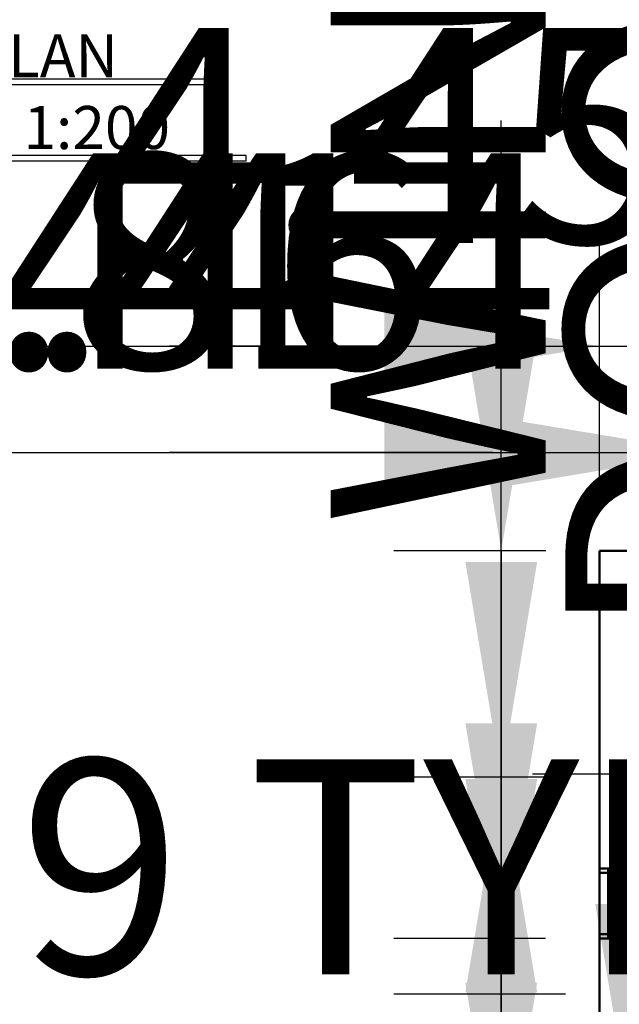
# Model space of a CAD drawing. Units: metres. Extents: x 782 to 1487, y 1262 to 7446.
# Tile 16 of 25: x 821.23 to 828.19, y 1302.06 to 1313.5. Entities that reach past the tile are written whole.
import ezdxf

# ---------------------------------------------------------------- set-up
doc = ezdxf.new("R2010")
doc.units = ezdxf.units.M
for name, color, linetype, lineweight in [('A-ANNO-DIMS', 2, 'Continuous', 18), ('A-ANNO-TEXT', 3, 'Continuous', 18), ('A-WALL', 7, 'Continuous', 50), ('C-PROP', 6, 'Continuous', 25)]:
    doc.layers.add(name, color=color, linetype=linetype, lineweight=lineweight)
doc.styles.get("Standard").update_dxf_attribs({"font": 'arial.ttf'})
doc.dimstyles.new('ISO-25', dxfattribs={"dimtxt": 2.5, "dimasz": 2.5, "dimexe": 1.25, "dimexo": 0.625, "dimtad": 1, "dimtxsty": 'Standard', "dimcen": 2.5, "dimadec": 0, "dimazin": 0, "dimtfac": 1, "dimtmove": 0, "dimatfit": 3, "dimfxl": 1, "dimarcsym": 0})

# ---------------------------------------------------------------- blocks, each defined once
blk = doc.blocks.new('*D5')
at = {"layer": 'A-ANNO-DIMS', "color": 0, "lineweight": -2, "transparency": 16777216}
for p, q in [((812.13, 1307.952), (812.13, 1310.955)), ((816.58, 1307.952), (816.58, 1310.955)), ((809.63, 1309.705), (807.13, 1309.705)), ((812.13, 1309.705), (816.58, 1309.705)), ((819.08, 1309.705), (829.443, 1309.705))]:
    blk.add_line(p, q, dxfattribs=at)
at = {"layer": 'A-ANNO-DIMS', "color": 0, "transparency": 16777216}
for points in [[(809.63, 1310.122), (809.63, 1309.289), (812.13, 1309.705)], [(819.08, 1310.122), (819.08, 1309.289), (816.58, 1309.705)]]:
    blk.add_solid(points, dxfattribs=at)
at = {"layer": 'Defpoints', "color": 0, "transparency": 16777216}
for p in [(816.58, 1309.705), (812.13, 1307.327), (816.58, 1307.327)]:
    blk.add_point(p, dxfattribs=at)
at = {"layer": 'A-ANNO-DIMS', "color": 0, "transparency": 16777216, "insert": (825.512, 1311.828), "char_height": 2.5, "attachment_point": 5}
blk.add_mtext('4,45', dxfattribs=at)
blk = doc.blocks.new('*D7')
at = {"layer": 'A-ANNO-DIMS', "color": 0, "lineweight": -2, "transparency": 16777216}
for p, q in [((827.962, 1307.952), (827.962, 1310.955)), ((832.412, 1307.952), (832.412, 1310.955)), ((825.462, 1309.705), (822.962, 1309.705)), ((827.962, 1309.705), (832.412, 1309.705)), ((834.912, 1309.705), (845.276, 1309.705))]:
    blk.add_line(p, q, dxfattribs=at)
at = {"layer": 'A-ANNO-DIMS', "color": 0, "transparency": 16777216}
for points in [[(825.462, 1310.122), (825.462, 1309.289), (827.962, 1309.705)], [(834.912, 1310.122), (834.912, 1309.289), (832.412, 1309.705)]]:
    blk.add_solid(points, dxfattribs=at)
at = {"layer": 'Defpoints', "color": 0, "transparency": 16777216}
for p in [(832.412, 1309.705), (827.962, 1307.327), (832.412, 1307.327)]:
    blk.add_point(p, dxfattribs=at)
at = {"layer": 'A-ANNO-DIMS', "color": 0, "transparency": 16777216, "insert": (841.344, 1311.828), "char_height": 2.5, "attachment_point": 5}
blk.add_mtext('4,45', dxfattribs=at)
blk = doc.blocks.new('*D20')
at = {"layer": 'A-ANNO-DIMS', "color": 0, "lineweight": -2, "transparency": 16777216}
for p, q in [((831.056, 1302.088), (831.056, 1337.678)), ((831.056, 1298.698), (831.056, 1299.588)), ((831.548, 1299.588), (832.306, 1299.588)), ((831.548, 1298.698), (832.306, 1298.698)), ((831.056, 1296.198), (831.056, 1293.698))]:
    blk.add_line(p, q, dxfattribs=at)
at = {"layer": 'A-ANNO-DIMS', "color": 0, "transparency": 16777216}
for points in [[(830.64, 1302.088), (831.473, 1302.088), (831.056, 1299.588)], [(830.64, 1296.198), (831.473, 1296.198), (831.056, 1298.698)]]:
    blk.add_solid(points, dxfattribs=at)
at = {"layer": 'Defpoints', "color": 0, "transparency": 16777216}
for p in [(830.923, 1299.588), (831.056, 1299.588), (830.923, 1298.698)]:
    blk.add_point(p, dxfattribs=at)
at = {"layer": 'A-ANNO-DIMS', "color": 0, "transparency": 16777216, "insert": (829.138, 1321.133), "char_height": 2.5, "attachment_point": 5, "rotation": 90}
blk.add_mtext('DOOR D1 0.89 TYP.', dxfattribs=at)
blk = doc.blocks.new('*D21')
at = {"layer": 'A-ANNO-DIMS', "color": 0, "lineweight": -2, "transparency": 16777216}
for p, q in [((827.576, 1298.565), (825.076, 1298.565)), ((830.076, 1298.565), (830.923, 1298.565)), ((833.423, 1298.565), (852.255, 1298.565)), ((830.076, 1298.073), (830.076, 1297.315)), ((830.923, 1298.073), (830.923, 1297.315))]:
    blk.add_line(p, q, dxfattribs=at)
at = {"layer": 'A-ANNO-DIMS', "color": 0, "transparency": 16777216}
for points in [[(827.576, 1298.981), (827.576, 1298.148), (830.076, 1298.565)], [(833.423, 1298.981), (833.423, 1298.148), (830.923, 1298.565)]]:
    blk.add_solid(points, dxfattribs=at)
at = {"layer": 'Defpoints', "color": 0, "transparency": 16777216}
for p in [(830.076, 1298.698), (830.923, 1298.698), (830.923, 1298.565)]:
    blk.add_point(p, dxfattribs=at)
at = {"layer": 'A-ANNO-DIMS', "color": 0, "transparency": 16777216, "insert": (844.089, 1300.466), "char_height": 2.5, "attachment_point": 5}
blk.add_mtext('0.85 TYP.', dxfattribs=at)
blk = doc.blocks.new('*D24')
at = {"layer": 'A-ANNO-DIMS', "color": 0, "lineweight": -2, "transparency": 16777216}
for p, q in [((811.209, 1294.423), (808.709, 1294.423)), ((813.709, 1294.423), (814.559, 1294.423)), ((817.059, 1294.423), (852.649, 1294.423)), ((813.709, 1293.926), (813.709, 1293.173)), ((814.559, 1293.926), (814.559, 1293.173))]:
    blk.add_line(p, q, dxfattribs=at)
at = {"layer": 'A-ANNO-DIMS', "color": 0, "transparency": 16777216}
for points in [[(811.209, 1294.84), (811.209, 1294.006), (813.709, 1294.423)], [(817.059, 1294.84), (817.059, 1294.006), (814.559, 1294.423)]]:
    blk.add_solid(points, dxfattribs=at)
at = {"layer": 'Defpoints', "color": 0, "transparency": 16777216}
for p in [(813.709, 1294.551), (814.559, 1294.551), (814.559, 1294.423)]:
    blk.add_point(p, dxfattribs=at)
at = {"layer": 'A-ANNO-DIMS', "color": 0, "transparency": 16777216, "insert": (836.104, 1296.342), "char_height": 2.5, "attachment_point": 5}
blk.add_mtext('DOOR D2 0.85 TYP.', dxfattribs=at)
blk = doc.blocks.new('*D26')
at = {"layer": 'A-ANNO-DIMS', "color": 0, "lineweight": -2, "transparency": 16777216}
for p, q in [((828.33, 1303.223), (828.33, 1342.718)), ((828.33, 1299.809), (828.33, 1300.723)), ((828.818, 1300.723), (829.58, 1300.723)), ((828.818, 1299.809), (829.58, 1299.809)), ((828.33, 1297.309), (828.33, 1294.809))]:
    blk.add_line(p, q, dxfattribs=at)
at = {"layer": 'A-ANNO-DIMS', "color": 0, "transparency": 16777216}
for points in [[(827.913, 1303.223), (828.747, 1303.223), (828.33, 1300.723)], [(827.913, 1297.309), (828.747, 1297.309), (828.33, 1299.809)]]:
    blk.add_solid(points, dxfattribs=at)
at = {"layer": 'Defpoints', "color": 0, "transparency": 16777216}
for p in [(828.193, 1300.723), (828.33, 1300.723), (828.193, 1299.809)]:
    blk.add_point(p, dxfattribs=at)
at = {"layer": 'A-ANNO-DIMS', "color": 0, "transparency": 16777216, "insert": (826.412, 1324.22), "char_height": 2.5, "attachment_point": 5, "rotation": 90}
blk.add_mtext('WINDOW W 0.91 TYP.', dxfattribs=at)
blk = doc.blocks.new('*D27')
at = {"layer": 'A-ANNO-DIMS', "color": 0, "lineweight": -2, "transparency": 16777216}
for p, q in [((825.463, 1299.672), (822.963, 1299.672)), ((827.963, 1299.672), (828.193, 1299.672)), ((830.693, 1299.672), (849.525, 1299.672)), ((827.963, 1299.184), (827.963, 1298.422)), ((828.193, 1299.184), (828.193, 1298.422))]:
    blk.add_line(p, q, dxfattribs=at)
at = {"layer": 'A-ANNO-DIMS', "color": 0, "transparency": 16777216}
for points in [[(825.463, 1300.088), (825.463, 1299.255), (827.963, 1299.672)], [(830.693, 1300.088), (830.693, 1299.255), (828.193, 1299.672)]]:
    blk.add_solid(points, dxfattribs=at)
at = {"layer": 'Defpoints', "color": 0, "transparency": 16777216}
for p in [(827.963, 1299.809), (828.193, 1299.809), (828.193, 1299.672)]:
    blk.add_point(p, dxfattribs=at)
at = {"layer": 'A-ANNO-DIMS', "color": 0, "transparency": 16777216, "insert": (841.359, 1301.574), "char_height": 2.5, "attachment_point": 5}
blk.add_mtext('0.23 TYP.', dxfattribs=at)
blk = doc.blocks.new('*D28')
at = {"layer": 'A-ANNO-DIMS', "color": 0, "lineweight": -2, "transparency": 16777216}
for p, q in [((832.55, 1308.281), (832.55, 1349.718)), ((832.55, 1304.867), (832.55, 1305.781)), ((833.038, 1305.781), (833.8, 1305.781)), ((833.038, 1304.867), (833.8, 1304.867)), ((832.55, 1302.367), (832.55, 1299.867))]:
    blk.add_line(p, q, dxfattribs=at)
at = {"layer": 'A-ANNO-DIMS', "color": 0, "transparency": 16777216}
for points in [[(832.134, 1308.281), (832.967, 1308.281), (832.55, 1305.781)], [(832.134, 1302.367), (832.967, 1302.367), (832.55, 1304.867)]]:
    blk.add_solid(points, dxfattribs=at)
at = {"layer": 'Defpoints', "color": 0, "transparency": 16777216}
for p in [(832.413, 1305.781), (832.55, 1305.781), (832.413, 1304.867)]:
    blk.add_point(p, dxfattribs=at)
at = {"layer": 'A-ANNO-DIMS', "color": 0, "transparency": 16777216, "insert": (830.632, 1330.25), "char_height": 2.5, "attachment_point": 5, "rotation": 90}
blk.add_mtext('WINDOW W1 0.91 TYP.', dxfattribs=at)
blk = doc.blocks.new('*D29')
at = {"layer": 'A-ANNO-DIMS', "color": 0, "lineweight": -2, "transparency": 16777216}
for p, q in [((829.683, 1304.73), (827.183, 1304.73)), ((832.183, 1304.73), (832.413, 1304.73)), ((834.913, 1304.73), (853.745, 1304.73)), ((832.183, 1304.242), (832.183, 1303.48)), ((832.413, 1304.242), (832.413, 1303.48))]:
    blk.add_line(p, q, dxfattribs=at)
at = {"layer": 'A-ANNO-DIMS', "color": 0, "transparency": 16777216}
for points in [[(829.683, 1305.146), (829.683, 1304.313), (832.183, 1304.73)], [(834.913, 1305.146), (834.913, 1304.313), (832.413, 1304.73)]]:
    blk.add_solid(points, dxfattribs=at)
at = {"layer": 'Defpoints', "color": 0, "transparency": 16777216}
for p in [(832.183, 1304.867), (832.413, 1304.867), (832.413, 1304.73)]:
    blk.add_point(p, dxfattribs=at)
at = {"layer": 'A-ANNO-DIMS', "color": 0, "transparency": 16777216, "insert": (845.579, 1306.632), "char_height": 2.5, "attachment_point": 5}
blk.add_mtext('0.23 TYP.', dxfattribs=at)
blk = doc.blocks.new('*D30')
at = {"layer": 'A-ANNO-DIMS', "color": 0, "lineweight": -2, "transparency": 16777216}
for p, q in [((792.059, 1301.411), (789.559, 1301.411)), ((794.559, 1301.411), (794.946, 1301.411)), ((797.446, 1301.411), (832.354, 1301.411)), ((794.559, 1300.844), (794.559, 1300.161)), ((794.946, 1300.844), (794.946, 1300.161))]:
    blk.add_line(p, q, dxfattribs=at)
at = {"layer": 'A-ANNO-DIMS', "color": 0, "transparency": 16777216}
for points in [[(792.059, 1301.827), (792.059, 1300.994), (794.559, 1301.411)], [(797.446, 1301.827), (797.446, 1300.994), (794.946, 1301.411)]]:
    blk.add_solid(points, dxfattribs=at)
at = {"layer": 'Defpoints', "color": 0, "transparency": 16777216}
for p in [(794.559, 1301.469), (794.946, 1301.469), (794.946, 1301.411)]:
    blk.add_point(p, dxfattribs=at)
at = {"layer": 'A-ANNO-DIMS', "color": 0, "transparency": 16777216, "insert": (816.15, 1303.33), "char_height": 2.5, "attachment_point": 5}
blk.add_mtext('COLUMN 0.39 TYP.', dxfattribs=at)
blk = doc.blocks.new('*D70')
at = {"layer": 'A-ANNO-DIMS', "color": 0, "lineweight": -2, "transparency": 16777216}
for p, q in [((812.13, 1307.952), (812.13, 1309.718)), ((812.573, 1307.953), (812.573, 1309.718)), ((809.63, 1308.468), (807.13, 1308.468)), ((812.13, 1308.468), (812.573, 1308.468)), ((815.073, 1308.468), (825.307, 1308.468))]:
    blk.add_line(p, q, dxfattribs=at)
at = {"layer": 'A-ANNO-DIMS', "color": 0, "transparency": 16777216}
for points in [[(809.63, 1308.884), (809.63, 1308.051), (812.13, 1308.468)], [(815.073, 1308.884), (815.073, 1308.051), (812.573, 1308.468)]]:
    blk.add_solid(points, dxfattribs=at)
at = {"layer": 'Defpoints', "color": 0, "transparency": 16777216}
for p in [(812.573, 1308.468), (812.13, 1307.327), (812.573, 1307.328)]:
    blk.add_point(p, dxfattribs=at)
at = {"layer": 'A-ANNO-DIMS', "color": 0, "transparency": 16777216, "insert": (821.44, 1310.369), "char_height": 2.5, "attachment_point": 5}
blk.add_mtext('0.44', dxfattribs=at)
blk = doc.blocks.new('*D71')
at = {"layer": 'A-ANNO-DIMS', "color": 0, "lineweight": -2, "transparency": 16777216}
for p, q in [((812.573, 1307.953), (812.573, 1309.718)), ((813.387, 1307.953), (813.387, 1309.718)), ((810.073, 1308.468), (807.573, 1308.468)), ((812.573, 1308.468), (813.387, 1308.468)), ((815.887, 1308.468), (828.063, 1308.468))]:
    blk.add_line(p, q, dxfattribs=at)
at = {"layer": 'A-ANNO-DIMS', "color": 0, "transparency": 16777216}
for points in [[(810.073, 1308.884), (810.073, 1308.051), (812.573, 1308.468)], [(815.887, 1308.884), (815.887, 1308.051), (813.387, 1308.468)]]:
    blk.add_solid(points, dxfattribs=at)
at = {"layer": 'Defpoints', "color": 0, "transparency": 16777216}
for p in [(813.387, 1308.468), (812.573, 1307.328), (813.387, 1307.328)]:
    blk.add_point(p, dxfattribs=at)
at = {"layer": 'A-ANNO-DIMS', "color": 0, "transparency": 16777216, "insert": (823.225, 1310.369), "char_height": 2.5, "attachment_point": 5}
blk.add_mtext('0.814', dxfattribs=at)
blk = doc.blocks.new('*D72')
at = {"layer": 'A-ANNO-DIMS', "color": 0, "lineweight": -2, "transparency": 16777216}
for p, q in [((813.387, 1307.953), (813.387, 1309.718)), ((813.85, 1307.722), (813.85, 1309.718)), ((810.887, 1308.468), (808.387, 1308.468)), ((813.387, 1308.468), (813.85, 1308.468)), ((816.35, 1308.468), (826.592, 1308.468))]:
    blk.add_line(p, q, dxfattribs=at)
at = {"layer": 'A-ANNO-DIMS', "color": 0, "transparency": 16777216}
for points in [[(810.887, 1308.884), (810.887, 1308.051), (813.387, 1308.468)], [(816.35, 1308.884), (816.35, 1308.051), (813.85, 1308.468)]]:
    blk.add_solid(points, dxfattribs=at)
at = {"layer": 'Defpoints', "color": 0, "transparency": 16777216}
for p in [(813.85, 1308.468), (813.387, 1307.328), (813.85, 1307.097)]:
    blk.add_point(p, dxfattribs=at)
at = {"layer": 'A-ANNO-DIMS', "color": 0, "transparency": 16777216, "insert": (822.721, 1310.369), "char_height": 2.5, "attachment_point": 5}
blk.add_mtext('0.46', dxfattribs=at)
blk = doc.blocks.new('*D77')
at = {"layer": 'A-ANNO-DIMS', "color": 0, "lineweight": -2, "transparency": 16777216}
for p, q in [((826.821, 1309.827), (826.821, 1312.327)), ((827.337, 1307.327), (825.571, 1307.327)), ((826.821, 1307.327), (826.821, 1304.697)), ((827.567, 1304.697), (825.571, 1304.697)), ((826.821, 1302.197), (826.821, 1291.911))]:
    blk.add_line(p, q, dxfattribs=at)
at = {"layer": 'A-ANNO-DIMS', "color": 0, "transparency": 16777216}
for points in [[(826.404, 1309.827), (827.238, 1309.827), (826.821, 1307.327)], [(826.404, 1302.197), (827.238, 1302.197), (826.821, 1304.697)]]:
    blk.add_solid(points, dxfattribs=at)
at = {"layer": 'Defpoints', "color": 0, "transparency": 16777216}
for p in [(827.962, 1307.327), (826.821, 1304.697), (828.192, 1304.697)]:
    blk.add_point(p, dxfattribs=at)
at = {"layer": 'A-ANNO-DIMS', "color": 0, "transparency": 16777216, "insert": (824.919, 1295.804), "char_height": 2.5, "attachment_point": 5, "rotation": 90}
blk.add_mtext('2.63', dxfattribs=at)
blk = doc.blocks.new('*D78')
at = {"layer": 'A-ANNO-DIMS', "color": 0, "lineweight": -2, "transparency": 16777216}
for p, q in [((826.821, 1307.197), (826.821, 1309.697)), ((827.567, 1304.697), (825.571, 1304.697)), ((826.821, 1304.697), (826.821, 1302.822)), ((827.336, 1302.822), (825.571, 1302.822)), ((826.821, 1300.322), (826.821, 1290.308))]:
    blk.add_line(p, q, dxfattribs=at)
at = {"layer": 'A-ANNO-DIMS', "color": 0, "transparency": 16777216}
for points in [[(826.404, 1307.197), (827.238, 1307.197), (826.821, 1304.697)], [(826.404, 1300.322), (827.238, 1300.322), (826.821, 1302.822)]]:
    blk.add_solid(points, dxfattribs=at)
at = {"layer": 'Defpoints', "color": 0, "transparency": 16777216}
for p in [(828.192, 1304.697), (826.821, 1302.822), (827.961, 1302.822)]:
    blk.add_point(p, dxfattribs=at)
at = {"layer": 'A-ANNO-DIMS', "color": 0, "transparency": 16777216, "insert": (824.919, 1294.065), "char_height": 2.5, "attachment_point": 5, "rotation": 90}
blk.add_mtext('1.88', dxfattribs=at)
blk = doc.blocks.new('*D79')
at = {"layer": 'A-ANNO-DIMS', "color": 0, "lineweight": -2, "transparency": 16777216}
for p, q in [((826.821, 1305.322), (826.821, 1307.822)), ((827.336, 1302.822), (825.571, 1302.822)), ((826.821, 1302.822), (826.821, 1302.177)), ((827.567, 1302.177), (825.571, 1302.177)), ((826.821, 1299.677), (826.821, 1289.444))]:
    blk.add_line(p, q, dxfattribs=at)
at = {"layer": 'A-ANNO-DIMS', "color": 0, "transparency": 16777216}
for points in [[(826.404, 1305.322), (827.238, 1305.322), (826.821, 1302.822)], [(826.404, 1299.677), (827.238, 1299.677), (826.821, 1302.177)]]:
    blk.add_solid(points, dxfattribs=at)
at = {"layer": 'Defpoints', "color": 0, "transparency": 16777216}
for p in [(827.961, 1302.822), (826.821, 1302.177), (828.192, 1302.177)]:
    blk.add_point(p, dxfattribs=at)
at = {"layer": 'A-ANNO-DIMS', "color": 0, "transparency": 16777216, "insert": (824.919, 1293.311), "char_height": 2.5, "attachment_point": 5, "rotation": 90}
blk.add_mtext('0.64', dxfattribs=at)
blk = doc.blocks.new('*D80')
at = {"layer": 'A-ANNO-DIMS', "color": 0, "lineweight": -2, "transparency": 16777216}
for p, q in [((826.821, 1304.677), (826.821, 1307.177)), ((827.567, 1302.177), (825.571, 1302.177)), ((826.821, 1302.177), (826.821, 1299.809)), ((827.338, 1299.809), (825.571, 1299.809)), ((826.821, 1297.309), (826.821, 1287.022))]:
    blk.add_line(p, q, dxfattribs=at)
at = {"layer": 'A-ANNO-DIMS', "color": 0, "transparency": 16777216}
for points in [[(826.404, 1304.677), (827.238, 1304.677), (826.821, 1302.177)], [(826.404, 1297.309), (827.238, 1297.309), (826.821, 1299.809)]]:
    blk.add_solid(points, dxfattribs=at)
at = {"layer": 'Defpoints', "color": 0, "transparency": 16777216}
for p in [(828.192, 1302.177), (826.821, 1299.809), (827.963, 1299.809)]:
    blk.add_point(p, dxfattribs=at)
at = {"layer": 'A-ANNO-DIMS', "color": 0, "transparency": 16777216, "insert": (824.919, 1290.916), "char_height": 2.5, "attachment_point": 5, "rotation": 90}
blk.add_mtext('2.37', dxfattribs=at)
blk = doc.blocks.new('*D81')
at = {"layer": 'A-ANNO-DIMS', "color": 0, "lineweight": -2, "transparency": 16777216}
for p, q in [((826.821, 1302.309), (826.821, 1304.809)), ((827.338, 1299.809), (825.571, 1299.809)), ((826.821, 1299.809), (826.821, 1298.647)), ((827.567, 1298.647), (825.571, 1298.647)), ((826.821, 1296.147), (826.821, 1286.141))]:
    blk.add_line(p, q, dxfattribs=at)
at = {"layer": 'A-ANNO-DIMS', "color": 0, "transparency": 16777216}
for points in [[(826.404, 1302.309), (827.238, 1302.309), (826.821, 1299.809)], [(826.404, 1296.147), (827.238, 1296.147), (826.821, 1298.647)]]:
    blk.add_solid(points, dxfattribs=at)
at = {"layer": 'Defpoints', "color": 0, "transparency": 16777216}
for p in [(827.963, 1299.809), (826.821, 1298.647), (828.192, 1298.647)]:
    blk.add_point(p, dxfattribs=at)
at = {"layer": 'A-ANNO-DIMS', "color": 0, "transparency": 16777216, "insert": (824.919, 1289.894), "char_height": 2.5, "attachment_point": 5, "rotation": 90}
blk.add_mtext('1.16', dxfattribs=at)
blk = doc.blocks.new('*D82')
at = {"layer": 'A-ANNO-DIMS', "color": 0, "lineweight": -2, "transparency": 16777216}
for p, q in [((826.821, 1301.147), (826.821, 1303.647)), ((827.567, 1298.647), (825.571, 1298.647)), ((826.821, 1298.647), (826.821, 1296.5)), ((827.339, 1296.5), (825.571, 1296.5)), ((826.821, 1294), (826.821, 1281.772))]:
    blk.add_line(p, q, dxfattribs=at)
at = {"layer": 'A-ANNO-DIMS', "color": 0, "transparency": 16777216}
for points in [[(826.404, 1301.147), (827.238, 1301.147), (826.821, 1298.647)], [(826.404, 1294), (827.238, 1294), (826.821, 1296.5)]]:
    blk.add_solid(points, dxfattribs=at)
at = {"layer": 'Defpoints', "color": 0, "transparency": 16777216}
for p in [(828.192, 1298.647), (826.821, 1296.5), (827.964, 1296.5)]:
    blk.add_point(p, dxfattribs=at)
at = {"layer": 'A-ANNO-DIMS', "color": 0, "transparency": 16777216, "insert": (824.941, 1286.636), "char_height": 2.5, "attachment_point": 5, "rotation": 90}
blk.add_mtext('2.147', dxfattribs=at)
blk = doc.blocks.new('*D94')
at = {"layer": 'A-ANNO-DIMS', "color": 0, "lineweight": -2, "transparency": 16777216}
for p, q in [((827.962, 1307.952), (827.962, 1309.718)), ((828.406, 1307.953), (828.406, 1309.718)), ((825.462, 1308.468), (822.962, 1308.468)), ((827.962, 1308.468), (828.406, 1308.468)), ((830.906, 1308.468), (841.139, 1308.468))]:
    blk.add_line(p, q, dxfattribs=at)
at = {"layer": 'A-ANNO-DIMS', "color": 0, "transparency": 16777216}
for points in [[(825.462, 1308.884), (825.462, 1308.051), (827.962, 1308.468)], [(830.906, 1308.884), (830.906, 1308.051), (828.406, 1308.468)]]:
    blk.add_solid(points, dxfattribs=at)
at = {"layer": 'Defpoints', "color": 0, "transparency": 16777216}
for p in [(828.406, 1308.468), (827.962, 1307.327), (828.406, 1307.328)]:
    blk.add_point(p, dxfattribs=at)
at = {"layer": 'A-ANNO-DIMS', "color": 0, "transparency": 16777216, "insert": (837.273, 1310.369), "char_height": 2.5, "attachment_point": 5}
blk.add_mtext('0.44', dxfattribs=at)
blk = doc.blocks.new('*D95')
at = {"layer": 'A-ANNO-DIMS', "color": 0, "lineweight": -2, "transparency": 16777216}
for p, q in [((828.406, 1307.953), (828.406, 1309.718)), ((829.22, 1307.953), (829.22, 1309.718)), ((825.906, 1308.468), (823.406, 1308.468)), ((828.406, 1308.468), (829.22, 1308.468)), ((831.72, 1308.468), (843.896, 1308.468))]:
    blk.add_line(p, q, dxfattribs=at)
at = {"layer": 'A-ANNO-DIMS', "color": 0, "transparency": 16777216}
for points in [[(825.906, 1308.884), (825.906, 1308.051), (828.406, 1308.468)], [(831.72, 1308.884), (831.72, 1308.051), (829.22, 1308.468)]]:
    blk.add_solid(points, dxfattribs=at)
at = {"layer": 'Defpoints', "color": 0, "transparency": 16777216}
for p in [(829.22, 1308.468), (828.406, 1307.328), (829.22, 1307.328)]:
    blk.add_point(p, dxfattribs=at)
at = {"layer": 'A-ANNO-DIMS', "color": 0, "transparency": 16777216, "insert": (839.058, 1310.369), "char_height": 2.5, "attachment_point": 5}
blk.add_mtext('0.814', dxfattribs=at)
blk = doc.blocks.new('*D96')
at = {"layer": 'A-ANNO-DIMS', "color": 0, "lineweight": -2, "transparency": 16777216}
for p, q in [((829.22, 1307.953), (829.22, 1309.718)), ((829.682, 1307.722), (829.682, 1309.718)), ((826.72, 1308.468), (824.22, 1308.468)), ((829.22, 1308.468), (829.682, 1308.468)), ((832.182, 1308.468), (842.425, 1308.468))]:
    blk.add_line(p, q, dxfattribs=at)
at = {"layer": 'A-ANNO-DIMS', "color": 0, "transparency": 16777216}
for points in [[(826.72, 1308.884), (826.72, 1308.051), (829.22, 1308.468)], [(832.182, 1308.884), (832.182, 1308.051), (829.682, 1308.468)]]:
    blk.add_solid(points, dxfattribs=at)
at = {"layer": 'Defpoints', "color": 0, "transparency": 16777216}
for p in [(829.682, 1308.468), (829.22, 1307.328), (829.682, 1307.097)]:
    blk.add_point(p, dxfattribs=at)
at = {"layer": 'A-ANNO-DIMS', "color": 0, "transparency": 16777216, "insert": (838.554, 1310.369), "char_height": 2.5, "attachment_point": 5}
blk.add_mtext('0.46', dxfattribs=at)

msp = doc.modelspace()

# ---------------------------------------------------------------- linework, layer by layer
at = {"layer": 'A-WALL'}
for p, q in [((827.9625, 1304.6974), (827.9625, 1307.3274)), ((827.9625, 1307.3274), (829.4525, 1307.3274)), ((827.9625, 1302.1774), (827.9625, 1304.6974)), ((827.9609, 1302.8221), (827.9609, 1303.6361)), ((827.9609, 1303.6361), (828.1909, 1303.6361)), ((827.9609, 1303.6361), (827.9609, 1303.5853)), ((828.0632, 1303.6361), (828.0632, 1302.8221)), ((828.1909, 1303.6361), (828.0759, 1303.6361)), ((828.0759, 1303.6361), (828.0759, 1302.8221)), ((828.0886, 1303.6361), (828.0886, 1302.8221)), ((828.1909, 1303.6361), (828.1909, 1302.8221)), ((827.9609, 1303.5853), (828.1909, 1303.5853)), ((827.9609, 1302.8221), (827.9609, 1302.8729)), ((827.9609, 1302.8729), (828.1909, 1302.8729)), ((828.1909, 1302.8221), (827.9609, 1302.8221)), ((827.9625, 1298.6474), (827.9625, 1302.1774))]:
    msp.add_line(p, q, dxfattribs=at)
at = {"layer": 'C-PROP'}
for p, q in [((818.4097, 1312.8097), (823.558, 1312.8097)), ((823.558, 1312.8097), (823.558, 1312.7398)), ((823.558, 1312.7398), (818.4097, 1312.7398)), ((818.7034, 1311.923), (823.8517, 1311.923)), ((823.8517, 1311.8532), (818.7034, 1311.8532)), ((823.8517, 1311.923), (823.8517, 1311.8532))]:
    msp.add_line(p, q, dxfattribs=at)

# ---------------------------------------------------------------- texts
at = {"layer": 'A-ANNO-TEXT', "insert": (819.087, 1314.1616), "char_height": 0.5, "attachment_point": 1}
msp.add_mtext_dynamic_manual_height_columns('\\PSITE PLAN\\PSCALE 1:200', width=6.191207, gutter_width=12.5, heights=[0], dxfattribs=at)

# ---------------------------------------------------------------- dimensions: what is measured, and where the dimension line sits
at = {"layer": 'A-ANNO-DIMS'}
for base, p1, p2, text, picture, middle in [((832.5503, 1305.7809), (832.4132, 1304.8669), (832.4132, 1305.7809), 'WINDOW W1 <> TYP.', '*D28', (830.6318, 1330.2497)), ((828.3302, 1300.7228), (828.1931, 1299.8088), (828.1931, 1300.7228), 'WINDOW W <> TYP.', '*D26', (826.4117, 1324.2204)), ((831.0564, 1299.5877), (830.923, 1298.6982), (830.923, 1299.5877), 'DOOR D1 <> TYP.', '*D20', (829.138, 1321.1327))]:
    dim = msp.add_linear_dim(base=base, p1=p1, p2=p2, angle=90, text=text, dimstyle='ISO-25', override={"dimdec": 2, "dimlfac": 1, "dimrnd": 0, "dimzin": 0, "dimdsep": 46, "dimlunit": 2}, dxfattribs=at)
    dim.commit()
    dim.dimension.update_dxf_attribs({"geometry": picture, "text_midpoint": middle})
for base, p1, p2, override, picture, middle in [((816.58, 1309.7054), (812.13, 1307.3274), (816.58, 1307.3274), {"dimclrd": 0, "dimclre": 0, "dimclrt": 0}, '*D5', (825.5116, 1311.8277)), ((832.4125, 1309.7054), (827.9625, 1307.3274), (832.4125, 1307.3274), {"dimclrd": 0, "dimclre": 0, "dimclrt": 0}, '*D7', (841.3441, 1311.8277)), ((812.5733, 1308.4676), (812.13, 1307.3274), (812.5733, 1307.3276), {"dimdec": 2, "dimlfac": 1, "dimrnd": 0, "dimzin": 0, "dimdsep": 46, "dimlunit": 2}, '*D70', (821.4401, 1310.369)), ((813.3873, 1308.4676), (812.5733, 1307.3276), (813.3873, 1307.3276), {"dimdec": 3, "dimlfac": 1, "dimrnd": 0, "dimzin": 0, "dimdsep": 46, "dimlunit": 2}, '*D71', (823.2253, 1310.369)), ((813.85, 1308.4676), (813.3873, 1307.3276), (813.85, 1307.0974), {"dimdec": 2, "dimlfac": 1, "dimrnd": 0, "dimzin": 0, "dimdsep": 46, "dimlunit": 2}, '*D72', (822.7211, 1310.369)), ((828.4057, 1308.4676), (827.9625, 1307.3274), (828.4057, 1307.3276), {"dimdec": 2, "dimlfac": 1, "dimrnd": 0, "dimzin": 0, "dimdsep": 46, "dimlunit": 2}, '*D94', (837.2725, 1310.369)), ((829.2197, 1308.4676), (828.4057, 1307.3276), (829.2197, 1307.3276), {"dimdec": 3, "dimlfac": 1, "dimrnd": 0, "dimzin": 0, "dimdsep": 46, "dimlunit": 2}, '*D95', (839.0577, 1310.369)), ((829.6825, 1308.4676), (829.2197, 1307.3276), (829.6825, 1307.0974), {"dimdec": 2, "dimlfac": 1, "dimrnd": 0, "dimzin": 0, "dimdsep": 46, "dimlunit": 2}, '*D96', (838.5536, 1310.369))]:
    dim = msp.add_linear_dim(base=base, p1=p1, p2=p2, dimstyle='ISO-25', override=override, dxfattribs=at)
    dim.commit()
    dim.dimension.update_dxf_attribs({"geometry": picture, "text_midpoint": middle})
for base, p1, p2, override, picture, middle in [((826.8209, 1304.6974), (827.9625, 1307.3274), (828.1925, 1304.6974), {"dimdec": 2, "dimlfac": 1, "dimrnd": 0, "dimzin": 0, "dimdsep": 46, "dimlunit": 2}, '*D77', (824.9186, 1295.8042)), ((826.8209, 1302.8221), (828.1925, 1304.6974), (827.9609, 1302.8221), {"dimdec": 2, "dimlfac": 1, "dimrnd": 0, "dimzin": 0, "dimdsep": 46, "dimlunit": 2}, '*D78', (824.9195, 1294.0652)), ((826.8209, 1302.1774), (827.9609, 1302.8221), (828.1925, 1302.1774), {"dimdec": 2, "dimlfac": 1, "dimrnd": 0, "dimzin": 0, "dimdsep": 46, "dimlunit": 2}, '*D79', (824.9195, 1293.3106)), ((826.8209, 1299.8088), (828.1925, 1302.1774), (827.9631, 1299.8088), {"dimdec": 2, "dimlfac": 1, "dimrnd": 0, "dimzin": 0, "dimdsep": 46, "dimlunit": 2}, '*D80', (824.9186, 1290.9156)), ((826.8209, 1298.6474), (827.9631, 1299.8088), (828.1925, 1298.6474), {"dimdec": 2, "dimlfac": 1, "dimrnd": 0, "dimzin": 0, "dimdsep": 46, "dimlunit": 2}, '*D81', (824.9195, 1289.894)), ((826.8209, 1296.5004), (828.1925, 1298.6474), (827.9641, 1296.5004), {"dimdec": 3, "dimlfac": 1, "dimrnd": 0, "dimzin": 0, "dimdsep": 46, "dimlunit": 2}, '*D82', (824.9408, 1286.636))]:
    dim = msp.add_linear_dim(base=base, p1=p1, p2=p2, angle=90, dimstyle='ISO-25', override=override, dxfattribs=at)
    dim.commit()
    dim.dimension.update_dxf_attribs({"geometry": picture, "text_midpoint": middle})
for base, p1, p2, text, picture, middle in [((832.4132, 1304.7298), (832.1832, 1304.8669), (832.4132, 1304.8669), '<> TYP.', '*D29', (845.5791, 1306.6321)), ((794.9459, 1301.4107), (794.559, 1301.4687), (794.9459, 1301.4687), 'COLUMN <> TYP.', '*D30', (816.1499, 1303.33)), ((828.1931, 1299.6717), (827.9631, 1299.8088), (828.1931, 1299.8088), '<> TYP.', '*D27', (841.359, 1301.574)), ((814.5592, 1294.4231), (813.7086, 1294.5507), (814.5592, 1294.5507), 'DOOR D2 <> TYP.', '*D24', (836.1042, 1296.3416)), ((830.923, 1298.5648), (830.0763, 1298.6982), (830.923, 1298.6982), '<> TYP.', '*D21', (844.0889, 1300.4662))]:
    dim = msp.add_linear_dim(base=base, p1=p1, p2=p2, text=text, dimstyle='ISO-25', override={"dimdec": 2, "dimlfac": 1, "dimrnd": 0, "dimzin": 0, "dimdsep": 46, "dimlunit": 2}, dxfattribs=at)
    dim.commit()
    dim.dimension.update_dxf_attribs({"geometry": picture, "text_midpoint": middle})

doc.saveas('drawing.dxf')
